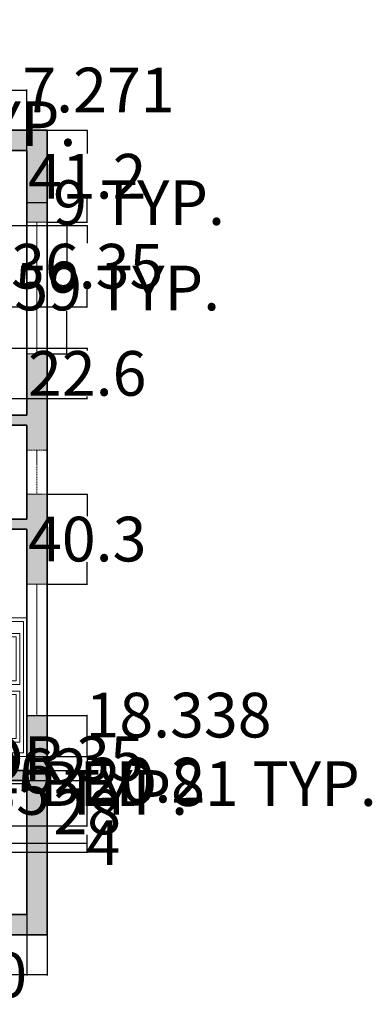
# Model space of a CAD drawing. Units: inches. Extents: x 305 to 776, y 38 to 479.
# Tile 14 of 14: x 618 to 776, y 38 to 479. Entities that reach past the tile are written whole.
import ezdxf

# ---------------------------------------------------------------- set-up
doc = ezdxf.new("R2010")
doc.units = ezdxf.units.IN
doc.header["$MEASUREMENT"] = 0
doc.linetypes.add('DASHED', pattern=[0.75, 0.5, -0.25])
for name, color, linetype, lineweight in [('A-ANNO-DIMS', 2, 'Continuous', 18), ('A-FURN', 8, 'Continuous', 18), ('A-GLAZ', 4, 'Continuous', 20), ('A-GLAZ-OVHD', 4, 'DASHED', 18), ('A-WALL', 7, 'Continuous', 35), ('A-WALL-PATT', 252, 'Continuous', 13)]:
    doc.layers.add(name, color=color, linetype=linetype, lineweight=lineweight)
doc.styles.get("Standard").update_dxf_attribs({"font": 'arial.ttf'})
doc.dimstyles.get("Standard").update_dxf_attribs({"dimtxt": 20, "dimasz": 0.18, "dimexe": 0.18, "dimexo": 0.0625, "dimgap": 0.09, "dimtad": 0, "dimtih": 1, "dimtoh": 1, "dimdec": 4, "dimzin": 0, "dimdsep": 46, "dimtxsty": 'Standard', "dimcen": 0.09, "dimadec": 0, "dimazin": 0, "dimtfac": 1, "dimtdec": 4, "dimtofl": 0, "dimtmove": 0, "dimatfit": 3, "dimfxl": 1, "dimtolj": 1, "dimtzin": 0, "dimarcsym": 0})

# ---------------------------------------------------------------- blocks, each defined once
blk = doc.blocks.new('W1')
blk.add_line((867.01, 338.44), (847.41, 338.44))
blk.add_lwpolyline([(847.41, 333.94), (867.01, 333.94), (867.01, 342.94), (847.41, 342.94)], close=True)
blk = doc.blocks.new('BED')
for p, q in [((1579.44, 254.58), (1564.49, 243.77)), ((1564.49, 243.77), (1579.44, 254.58)), ((1626.49, 254.58), (1579.44, 254.58)), ((1579.44, 254.58), (1579.44, 243.77)), ((1626.49, 253.76), (1579.44, 253.76)), ((1579.44, 243.77), (1564.49, 243.77))]:
    blk.add_line(p, q)
for points in [[(1626.49, 214.2), (1564.49, 214.2), (1564.49, 294.96), (1626.49, 294.96)], [(1624.92, 215.77), (1566.06, 215.77), (1566.06, 293.39), (1624.92, 293.39)], [(1594.24, 275.39), (1571.42, 275.39), (1571.42, 291.78), (1594.24, 291.78)], [(1620.04, 275.39), (1597.22, 275.39), (1597.22, 291.78), (1620.04, 291.78)], [(1592.67, 276.96), (1572.99, 276.96), (1572.99, 290.21), (1592.67, 290.21)], [(1618.47, 276.96), (1598.79, 276.96), (1598.79, 290.21), (1618.47, 290.21)]]:
    blk.add_lwpolyline(points, close=True)
blk = doc.blocks.new('W3')
for p, q in [((867.01, 308.31), (847.41, 308.31)), ((886.61, 308.31), (867.01, 308.31)), ((906.21, 308.31), (886.61, 308.31))]:
    blk.add_line(p, q)
for points in [[(867.01, 312.81), (847.41, 312.81), (847.41, 303.81), (867.01, 303.81)], [(886.61, 312.81), (867.01, 312.81)], [(886.61, 303.81), (906.21, 303.81), (906.21, 312.81), (886.61, 312.81)], [(867.01, 303.81), (886.61, 303.81)]]:
    blk.add_lwpolyline(points)
blk = doc.blocks.new('*D17')
at = {"layer": 'A-ANNO-DIMS', "color": 0, "lineweight": -2, "transparency": 16777216}
for p, q in [((476.73, 138.32), (476.73, 132.89)), ((512.13, 138.32), (512.13, 132.89)), ((476.91, 133.07), (511.95, 133.07)), ((512.13, 133.07), (512.31, 133.07))]:
    blk.add_line(p, q, dxfattribs=at)
at = {"layer": 'A-ANNO-DIMS', "color": 0, "transparency": 16777216}
for points in [[(476.91, 133.1), (476.91, 133.04), (476.73, 133.07)], [(511.95, 133.1), (511.95, 133.04), (512.13, 133.07)]]:
    blk.add_solid(points, dxfattribs=at)
at = {"layer": 'Defpoints', "color": 0, "transparency": 16777216}
for p in [(476.73, 138.38), (512.13, 138.38), (512.13, 133.07)]:
    blk.add_point(p, dxfattribs=at)
at = {"layer": 'A-ANNO-DIMS', "color": 0, "transparency": 16777216, "insert": (606.37, 133.07), "char_height": 20, "attachment_point": 5}
blk.add_mtext('\\A1;DOOR 35 TYP.', dxfattribs=at)
blk = doc.blocks.new('*D21')
at = {"layer": 'A-ANNO-DIMS', "color": 0, "lineweight": -2, "transparency": 16777216}
for p, q in [((403.93, 142.94), (403.93, 148.37)), ((404.11, 148.19), (439.15, 148.19)), ((439.33, 142.94), (439.33, 148.37)), ((439.33, 148.19), (439.51, 148.19))]:
    blk.add_line(p, q, dxfattribs=at)
at = {"layer": 'A-ANNO-DIMS', "color": 0, "transparency": 16777216}
for points in [[(404.11, 148.22), (404.11, 148.16), (403.93, 148.19)], [(439.15, 148.22), (439.15, 148.16), (439.33, 148.19)]]:
    blk.add_solid(points, dxfattribs=at)
at = {"layer": 'Defpoints', "color": 0, "transparency": 16777216}
for p in [(439.33, 148.19), (403.93, 142.88), (439.33, 142.88)]:
    blk.add_point(p, dxfattribs=at)
at = {"layer": 'A-ANNO-DIMS', "color": 0, "transparency": 16777216, "insert": (560.63, 148.19), "char_height": 20, "attachment_point": 5}
blk.add_mtext('\\A1;DOUBLE DOOR 35', dxfattribs=at)
blk = doc.blocks.new('*D23')
at = {"layer": 'A-ANNO-DIMS', "color": 0, "lineweight": -2, "transparency": 16777216}
for p, q in [((481.33, 429.44), (481.33, 432.5)), ((481.51, 432.32), (500.75, 432.32)), ((500.93, 429.44), (500.93, 432.5)), ((500.93, 432.32), (501.11, 432.32))]:
    blk.add_line(p, q, dxfattribs=at)
at = {"layer": 'A-ANNO-DIMS', "color": 0, "transparency": 16777216}
for points in [[(481.51, 432.35), (481.51, 432.29), (481.33, 432.32)], [(500.75, 432.35), (500.75, 432.29), (500.93, 432.32)]]:
    blk.add_solid(points, dxfattribs=at)
at = {"layer": 'Defpoints', "color": 0, "transparency": 16777216}
for p in [(500.93, 432.32), (481.33, 429.38), (500.93, 429.38)]:
    blk.add_point(p, dxfattribs=at)
at = {"layer": 'A-ANNO-DIMS', "color": 0, "transparency": 16777216, "insert": (575.13, 432.32), "char_height": 20, "attachment_point": 5}
blk.add_mtext('\\A1;W1 20 TYP.', dxfattribs=at)
blk = doc.blocks.new('*D27')
at = {"layer": 'A-ANNO-DIMS', "color": 0, "lineweight": -2, "transparency": 16777216}
for p, q in [((630.7, 388.18), (639.63, 388.18)), ((639.45, 388), (639.45, 369.09)), ((639.45, 329.56), (639.45, 348.47)), ((630.7, 329.38), (639.63, 329.38))]:
    blk.add_line(p, q, dxfattribs=at)
at = {"layer": 'A-ANNO-DIMS', "color": 0, "transparency": 16777216}
for points in [[(639.42, 388), (639.48, 388), (639.45, 388.18)], [(639.42, 329.56), (639.48, 329.56), (639.45, 329.38)]]:
    blk.add_solid(points, dxfattribs=at)
at = {"layer": 'Defpoints', "color": 0, "transparency": 16777216}
for p in [(630.63, 388.18), (630.63, 329.38), (639.45, 329.38)]:
    blk.add_point(p, dxfattribs=at)
at = {"layer": 'A-ANNO-DIMS', "color": 0, "transparency": 16777216, "insert": (639.45, 358.78), "char_height": 20, "attachment_point": 5}
blk.add_mtext('\\A1;W3 59 TYP.', dxfattribs=at)
blk = doc.blocks.new('*D28')
at = {"layer": 'A-ANNO-DIMS', "color": 0, "lineweight": -2, "transparency": 16777216}
for p, q in [((621.63, 388.24), (621.63, 397.18)), ((621.81, 397), (630.45, 397)), ((630.63, 388.24), (630.63, 397.18)), ((630.63, 397), (630.81, 397))]:
    blk.add_line(p, q, dxfattribs=at)
at = {"layer": 'A-ANNO-DIMS', "color": 0, "transparency": 16777216}
for points in [[(621.81, 397.03), (621.81, 396.97), (621.63, 397)], [(630.45, 397.03), (630.45, 396.97), (630.63, 397)]]:
    blk.add_solid(points, dxfattribs=at)
at = {"layer": 'Defpoints', "color": 0, "transparency": 16777216}
for p in [(630.63, 397), (621.63, 388.18), (630.63, 388.18)]:
    blk.add_point(p, dxfattribs=at)
at = {"layer": 'A-ANNO-DIMS', "color": 0, "transparency": 16777216, "insert": (671.81, 397), "char_height": 20, "attachment_point": 5}
blk.add_mtext('\\A1;9 TYP.', dxfattribs=at)
blk = doc.blocks.new('*D29')
at = {"layer": 'A-ANNO-DIMS', "color": 0, "lineweight": -2, "transparency": 16777216}
for p, q in [((540.87, 149.08), (540.87, 136.85)), ((621.63, 149.08), (621.63, 136.85)), ((541.05, 137.03), (621.45, 137.03)), ((621.63, 137.03), (621.81, 137.03))]:
    blk.add_line(p, q, dxfattribs=at)
at = {"layer": 'A-ANNO-DIMS', "color": 0, "transparency": 16777216}
for points in [[(541.05, 137.06), (541.05, 137), (540.87, 137.03)], [(621.45, 137.06), (621.45, 137), (621.63, 137.03)]]:
    blk.add_solid(points, dxfattribs=at)
at = {"layer": 'Defpoints', "color": 0, "transparency": 16777216}
for p in [(540.87, 149.14), (621.63, 149.14), (621.63, 137.03)]:
    blk.add_point(p, dxfattribs=at)
at = {"layer": 'A-ANNO-DIMS', "color": 0, "transparency": 16777216, "insert": (702.74, 137.03), "char_height": 20, "attachment_point": 5}
blk.add_mtext('\\A1;BED 81 TYP.', dxfattribs=at)
blk = doc.blocks.new('*D45')
at = {"layer": 'A-ANNO-DIMS', "color": 0, "lineweight": -2, "transparency": 16777216}
for p, q in [((390.63, 69.32), (390.63, 51.2)), ((630.63, 69.32), (630.63, 51.2)), ((390.81, 51.38), (488.31, 51.38)), ((630.45, 51.38), (532.95, 51.38))]:
    blk.add_line(p, q, dxfattribs=at)
at = {"layer": 'A-ANNO-DIMS', "color": 0, "transparency": 16777216}
for points in [[(390.81, 51.41), (390.81, 51.35), (390.63, 51.38)], [(630.45, 51.41), (630.45, 51.35), (630.63, 51.38)]]:
    blk.add_solid(points, dxfattribs=at)
at = {"layer": 'Defpoints', "color": 0, "transparency": 16777216}
for p in [(390.63, 69.38), (630.63, 69.38), (630.63, 51.38)]:
    blk.add_point(p, dxfattribs=at)
at = {"layer": 'A-ANNO-DIMS', "color": 0, "transparency": 16777216, "insert": (510.63, 51.38), "char_height": 20, "attachment_point": 5}
blk.add_mtext('\\A1;240', dxfattribs=at)
blk = doc.blocks.new('*D48')
at = {"layer": 'A-ANNO-DIMS', "color": 0, "lineweight": -2, "transparency": 16777216}
for p, q in [((404, 138.38), (648.81, 138.38)), ((648.63, 138.38), (648.63, 138.56)), ((648.63, 138.56), (648.81, 138.56)), ((648.63, 118.36), (648.63, 138.2)), ((399.7, 118.18), (648.81, 118.18))]:
    blk.add_line(p, q, dxfattribs=at)
at = {"layer": 'A-ANNO-DIMS', "color": 0, "transparency": 16777216}
for points in [[(648.6, 138.2), (648.66, 138.2), (648.63, 138.38)], [(648.6, 118.36), (648.66, 118.36), (648.63, 118.18)]]:
    blk.add_solid(points, dxfattribs=at)
at = {"layer": 'Defpoints', "color": 0, "transparency": 16777216}
for p in [(403.93, 138.38), (648.63, 138.38), (399.63, 118.18)]:
    blk.add_point(p, dxfattribs=at)
at = {"layer": 'A-ANNO-DIMS', "color": 0, "transparency": 16777216, "insert": (674.95, 138.56), "char_height": 20, "attachment_point": 5}
blk.add_mtext('\\A1;20.2', dxfattribs=at)
blk = doc.blocks.new('*D49')
at = {"layer": 'A-ANNO-DIMS', "color": 0, "lineweight": -2, "transparency": 16777216}
for p, q in [((399.7, 331.88), (648.81, 331.88)), ((648.63, 331.7), (648.63, 330.88)), ((399.7, 309.28), (648.81, 309.28)), ((648.63, 309.46), (648.63, 310.28))]:
    blk.add_line(p, q, dxfattribs=at)
at = {"layer": 'A-ANNO-DIMS', "color": 0, "transparency": 16777216}
for points in [[(648.6, 331.7), (648.66, 331.7), (648.63, 331.88)], [(648.6, 309.46), (648.66, 309.46), (648.63, 309.28)]]:
    blk.add_solid(points, dxfattribs=at)
at = {"layer": 'Defpoints', "color": 0, "transparency": 16777216}
for p in [(399.63, 331.88), (648.63, 331.88), (399.63, 309.28)]:
    blk.add_point(p, dxfattribs=at)
at = {"layer": 'A-ANNO-DIMS', "color": 0, "transparency": 16777216, "insert": (648.63, 320.58), "char_height": 20, "attachment_point": 5}
blk.add_mtext('\\A1;22.6', dxfattribs=at)
blk = doc.blocks.new('*D51')
at = {"layer": 'A-ANNO-DIMS', "color": 0, "lineweight": -2, "transparency": 16777216}
for p, q in [((621.7, 167.48), (648.81, 167.48)), ((648.63, 167.48), (648.63, 167.66)), ((648.63, 167.66), (648.81, 167.66)), ((648.63, 149.32), (648.63, 167.3)), ((621.7, 149.14), (648.81, 149.14))]:
    blk.add_line(p, q, dxfattribs=at)
at = {"layer": 'A-ANNO-DIMS', "color": 0, "transparency": 16777216}
for points in [[(648.6, 167.3), (648.66, 167.3), (648.63, 167.48)], [(648.6, 149.32), (648.66, 149.32), (648.63, 149.14)]]:
    blk.add_solid(points, dxfattribs=at)
at = {"layer": 'Defpoints', "color": 0, "transparency": 16777216}
for p in [(621.63, 167.48), (648.63, 167.48), (621.63, 149.14)]:
    blk.add_point(p, dxfattribs=at)
at = {"layer": 'A-ANNO-DIMS', "color": 0, "transparency": 16777216, "insert": (689.5, 167.66), "char_height": 20, "attachment_point": 5}
blk.add_mtext('\\A1;18.338', dxfattribs=at)
blk = doc.blocks.new('*D52')
at = {"layer": 'A-ANNO-DIMS', "color": 0, "lineweight": -2, "transparency": 16777216}
for p, q in [((630.7, 266.58), (648.81, 266.58)), ((648.63, 266.4), (648.63, 256.74)), ((648.63, 226.46), (648.63, 236.12)), ((630.7, 226.28), (648.81, 226.28))]:
    blk.add_line(p, q, dxfattribs=at)
at = {"layer": 'A-ANNO-DIMS', "color": 0, "transparency": 16777216}
for points in [[(648.6, 266.4), (648.66, 266.4), (648.63, 266.58)], [(648.6, 226.46), (648.66, 226.46), (648.63, 226.28)]]:
    blk.add_solid(points, dxfattribs=at)
at = {"layer": 'Defpoints', "color": 0, "transparency": 16777216}
for p in [(630.63, 266.58), (648.63, 266.58), (630.63, 226.28)]:
    blk.add_point(p, dxfattribs=at)
at = {"layer": 'A-ANNO-DIMS', "color": 0, "transparency": 16777216, "insert": (648.63, 246.43), "char_height": 20, "attachment_point": 5}
blk.add_mtext('\\A1;40.3', dxfattribs=at)
blk = doc.blocks.new('*D53')
at = {"layer": 'A-ANNO-DIMS', "color": 0, "lineweight": -2, "transparency": 16777216}
for p, q in [((630.7, 429.38), (648.81, 429.38)), ((648.63, 429.2), (648.63, 418.91)), ((648.63, 388.36), (648.63, 398.65)), ((630.7, 388.18), (648.81, 388.18))]:
    blk.add_line(p, q, dxfattribs=at)
at = {"layer": 'A-ANNO-DIMS', "color": 0, "transparency": 16777216}
for points in [[(648.6, 429.2), (648.66, 429.2), (648.63, 429.38)], [(648.6, 388.36), (648.66, 388.36), (648.63, 388.18)]]:
    blk.add_solid(points, dxfattribs=at)
at = {"layer": 'Defpoints', "color": 0, "transparency": 16777216}
for p in [(630.63, 429.38), (630.63, 388.18), (648.63, 388.18)]:
    blk.add_point(p, dxfattribs=at)
at = {"layer": 'A-ANNO-DIMS', "color": 0, "transparency": 16777216, "insert": (648.63, 408.78), "char_height": 20, "attachment_point": 5}
blk.add_mtext('\\A1;41.2', dxfattribs=at)
blk = doc.blocks.new('*D56')
at = {"layer": 'A-ANNO-DIMS', "color": 0, "lineweight": -2, "transparency": 16777216}
for p, q in [((591.63, 78.32), (591.63, 51.2)), ((621.63, 78.32), (621.63, 51.2)), ((591.81, 51.38), (592.26, 51.38)), ((621.45, 51.38), (621.01, 51.38))]:
    blk.add_line(p, q, dxfattribs=at)
at = {"layer": 'A-ANNO-DIMS', "color": 0, "transparency": 16777216}
for points in [[(591.81, 51.41), (591.81, 51.35), (591.63, 51.38)], [(621.45, 51.41), (621.45, 51.35), (621.63, 51.38)]]:
    blk.add_solid(points, dxfattribs=at)
at = {"layer": 'Defpoints', "color": 0, "transparency": 16777216}
for p in [(591.63, 78.38), (621.63, 78.38), (621.63, 51.38)]:
    blk.add_point(p, dxfattribs=at)
at = {"layer": 'A-ANNO-DIMS', "color": 0, "transparency": 16777216, "insert": (606.63, 51.38), "char_height": 20, "attachment_point": 5}
blk.add_mtext('\\A1;30', dxfattribs=at)
blk = doc.blocks.new('*D57')
at = {"layer": 'A-ANNO-DIMS', "color": 0, "lineweight": -2, "transparency": 16777216}
for p, q in [((591.7, 138.38), (648.81, 138.38)), ((648.63, 138.2), (648.63, 134.68)), ((591.7, 110.38), (648.81, 110.38)), ((648.63, 110.56), (648.63, 114.08))]:
    blk.add_line(p, q, dxfattribs=at)
at = {"layer": 'A-ANNO-DIMS', "color": 0, "transparency": 16777216}
for points in [[(648.6, 138.2), (648.66, 138.2), (648.63, 138.38)], [(648.6, 110.56), (648.66, 110.56), (648.63, 110.38)]]:
    blk.add_solid(points, dxfattribs=at)
at = {"layer": 'Defpoints', "color": 0, "transparency": 16777216}
for p in [(591.63, 138.38), (591.63, 110.38), (648.63, 110.38)]:
    blk.add_point(p, dxfattribs=at)
at = {"layer": 'A-ANNO-DIMS', "color": 0, "transparency": 16777216, "insert": (648.63, 124.38), "char_height": 20, "attachment_point": 5}
blk.add_mtext('\\A1;28', dxfattribs=at)
blk = doc.blocks.new('*D59')
at = {"layer": 'A-ANNO-DIMS', "color": 0, "lineweight": -2, "transparency": 16777216}
for p, q in [((591.7, 110.38), (648.81, 110.38)), ((648.63, 110.38), (648.63, 110.56)), ((648.63, 110.56), (648.81, 110.56)), ((648.63, 106.56), (648.63, 110.2)), ((591.7, 106.38), (648.81, 106.38))]:
    blk.add_line(p, q, dxfattribs=at)
at = {"layer": 'A-ANNO-DIMS', "color": 0, "transparency": 16777216}
for points in [[(648.6, 110.2), (648.66, 110.2), (648.63, 110.38)], [(648.6, 106.56), (648.66, 106.56), (648.63, 106.38)]]:
    blk.add_solid(points, dxfattribs=at)
at = {"layer": 'Defpoints', "color": 0, "transparency": 16777216}
for p in [(591.63, 110.38), (648.63, 110.38), (591.63, 106.38)]:
    blk.add_point(p, dxfattribs=at)
at = {"layer": 'A-ANNO-DIMS', "color": 0, "transparency": 16777216, "insert": (655.82, 110.56), "char_height": 20, "attachment_point": 5}
blk.add_mtext('\\A1;4', dxfattribs=at)
blk = doc.blocks.new('*D64')
at = {"layer": 'A-ANNO-DIMS', "color": 0, "lineweight": -2, "transparency": 16777216}
for p, q in [((400.62, 386.71), (648.81, 386.71)), ((648.63, 386.53), (648.63, 378.84)), ((648.63, 350.53), (648.63, 358.22)), ((400.62, 350.35), (648.81, 350.35))]:
    blk.add_line(p, q, dxfattribs=at)
at = {"layer": 'A-ANNO-DIMS', "color": 0, "transparency": 16777216}
for points in [[(648.6, 386.53), (648.66, 386.53), (648.63, 386.71)], [(648.6, 350.53), (648.66, 350.53), (648.63, 350.35)]]:
    blk.add_solid(points, dxfattribs=at)
at = {"layer": 'Defpoints', "color": 0, "transparency": 16777216}
for p in [(400.56, 386.71), (648.63, 386.71), (400.56, 350.35)]:
    blk.add_point(p, dxfattribs=at)
at = {"layer": 'A-ANNO-DIMS', "color": 0, "transparency": 16777216, "insert": (648.63, 368.53), "char_height": 20, "attachment_point": 5}
blk.add_mtext('\\A1;36.35', dxfattribs=at)
blk = doc.blocks.new('*D68')
at = {"layer": 'A-ANNO-DIMS', "color": 0, "lineweight": -2, "transparency": 16777216}
for p, q in [((614.36, 420.44), (614.36, 447.56)), ((614.54, 447.38), (621.45, 447.38)), ((621.63, 420.44), (621.63, 447.56)), ((621.63, 447.38), (621.81, 447.38))]:
    blk.add_line(p, q, dxfattribs=at)
at = {"layer": 'A-ANNO-DIMS', "color": 0, "transparency": 16777216}
for points in [[(614.54, 447.41), (614.54, 447.35), (614.36, 447.38)], [(621.45, 447.41), (621.45, 447.35), (621.63, 447.38)]]:
    blk.add_solid(points, dxfattribs=at)
at = {"layer": 'Defpoints', "color": 0, "transparency": 16777216}
for p in [(621.63, 447.38), (614.36, 420.38), (621.63, 420.38)]:
    blk.add_point(p, dxfattribs=at)
at = {"layer": 'A-ANNO-DIMS', "color": 0, "transparency": 16777216, "insert": (653.64, 447.38), "char_height": 20, "attachment_point": 5}
blk.add_mtext('\\A1;7.271', dxfattribs=at)
blk = doc.blocks.new('*D69')
at = {"layer": 'A-ANNO-DIMS', "color": 0, "lineweight": -2, "transparency": 16777216}
for p, q in [((621.7, 149.14), (648.81, 149.14)), ((648.63, 148.96), (648.63, 143.06)), ((621.7, 142.88), (648.81, 142.88)), ((648.63, 142.7), (648.45, 142.7)), ((648.63, 142.88), (648.63, 142.7))]:
    blk.add_line(p, q, dxfattribs=at)
at = {"layer": 'A-ANNO-DIMS', "color": 0, "transparency": 16777216}
for points in [[(648.6, 148.96), (648.66, 148.96), (648.63, 149.14)], [(648.6, 143.06), (648.66, 143.06), (648.63, 142.88)]]:
    blk.add_solid(points, dxfattribs=at)
at = {"layer": 'Defpoints', "color": 0, "transparency": 16777216}
for p in [(621.63, 149.14), (621.63, 142.88), (648.63, 142.88)]:
    blk.add_point(p, dxfattribs=at)
at = {"layer": 'A-ANNO-DIMS', "color": 0, "transparency": 16777216, "insert": (614.67, 142.7), "char_height": 20, "attachment_point": 5}
blk.add_mtext('\\A1;6.262', dxfattribs=at)

msp = doc.modelspace()

# ---------------------------------------------------------------- hatches: boundary and pattern name
at = {"layer": 'A-WALL-PATT'}
h = msp.add_hatch(color=256, dxfattribs=at)
h.dxf.hatch_style = 1
h.paths.add_polyline_path([(481.3329, 429.382), (390.6329, 429.382), (390.6329, 398.067), (399.6329, 398.067), (399.6329, 420.382), (465.6329, 420.382), (465.6329, 331.882), (470.1329, 331.882), (470.1329, 355.882), (512.1329, 355.882), (512.1329, 337.282), (512.1329, 337.282), (515.8592, 337.282), (516.6329, 337.282), (516.6329, 360.382), (513.3171, 360.382), (470.1329, 360.382), (470.1329, 420.382), (481.3329, 420.382)])
h.paths.add_polyline_path([(630.6329, 429.382), (500.9329, 429.382), (500.9329, 420.382), (502.8693, 420.382), (512.1329, 420.382), (512.1329, 391.882), (516.6329, 391.882), (516.6329, 420.382), (621.6329, 420.382), (621.6329, 388.182), (630.6329, 388.182)])
h.paths.add_polyline_path([(630.6329, 329.382), (621.6329, 329.382), (621.6329, 301.882), (512.1329, 301.882), (512.1329, 297.382), (515.8592, 297.382), (557.6329, 297.382), (621.6329, 297.382), (621.6329, 286.182), (630.6329, 286.182)])
h.paths.add_polyline_path([(630.6329, 266.582), (621.6329, 266.582), (621.6329, 255.382), (589.1329, 255.382), (589.1329, 250.882), (621.6329, 250.882), (621.6329, 226.282), (630.6329, 226.282)])
h.paths.add_polyline_path([(630.6329, 167.482), (621.6329, 167.482), (621.6329, 149.1444), (621.6329, 142.882), (516.6329, 142.882), (516.6329, 261.982), (512.1329, 261.982), (512.1329, 138.382), (621.6329, 138.382), (621.6329, 78.382), (512.1329, 78.382), (512.1329, 69.382), (630.6329, 69.382)])
h.paths.add_polyline_path([(464.1329, 138.382), (476.7329, 138.382), (476.7329, 142.1084), (476.7329, 142.882), (459.6329, 142.882), (459.6329, 78.382), (399.6329, 78.382), (399.6329, 98.582), (390.6329, 98.582), (390.6329, 69.382), (464.1329, 69.382)])
h.paths.add_polyline_path([(459.6329, 142.882), (439.3329, 142.882), (439.3329, 138.382), (459.6329, 138.382)], flags=17)
h.paths.add_polyline_path([(399.6329, 138.382), (403.9329, 138.382), (403.9329, 141.5545), (403.9329, 141.5545), (403.9329, 142.882), (399.6329, 142.882), (399.6329, 250.4819), (390.6329, 250.4819), (390.6329, 118.182), (399.6329, 118.182)])
h.paths.add_polyline_path([(399.6329, 331.882), (428.2629, 331.882), (428.2629, 336.382), (399.6329, 336.382), (399.6329, 358.697), (390.6329, 358.697), (390.6329, 309.2819), (399.6329, 309.2819)])

# ---------------------------------------------------------------- linework, layer by layer
at = {"layer": 'A-WALL'}
for p, q in [((621.6329, 420.382), (516.6329, 420.382)), ((621.6329, 336.382), (621.6329, 420.382)), ((621.6329, 301.882), (621.6329, 336.382)), ((621.6329, 301.882), (512.1329, 301.882)), ((621.6329, 297.382), (557.6329, 297.382)), ((621.6329, 297.382), (557.6329, 297.382)), ((621.6329, 255.382), (621.6329, 297.382)), ((621.6329, 255.382), (589.1329, 255.382)), ((621.6329, 250.882), (589.1329, 250.882)), ((621.6329, 142.882), (621.6329, 250.882)), ((621.6329, 142.882), (516.6329, 142.882)), ((621.6329, 138.382), (464.1329, 138.382)), ((621.6329, 78.382), (621.6329, 138.382)), ((512.1329, 78.382), (621.6329, 78.382))]:
    msp.add_line(p, q, dxfattribs=at)
msp.add_lwpolyline([(390.6329, 69.382), (630.6329, 69.382), (630.6329, 429.382), (390.6329, 429.382)], close=True, dxfattribs=at)

# ---------------------------------------------------------------- block references
at = {"layer": 'A-FURN', "rotation": 270}
msp.add_blockref('BED', (326.6739, 1775.6374), dxfattribs=at)
at = {"layer": 'A-GLAZ', "rotation": 270}
for p in [(317.8213, 1235.5942), (317.8213, 1073.6942)]:
    msp.add_blockref('W3', p, dxfattribs=at)
at = {"layer": 'A-GLAZ-OVHD', "rotation": 90}
msp.add_blockref('W1', (964.5758, -580.8301), dxfattribs=at)

# ---------------------------------------------------------------- dimensions: what is measured, and where the dimension line sits
at = {"layer": 'A-ANNO-DIMS'}
for base, p1, p2, text, picture, middle in [((500.9329, 432.322), (481.3329, 429.382), (500.9329, 429.382), 'W1 <> TYP.', '*D23', (575.1251, 432.322)), ((630.6329, 397.002), (621.6329, 388.182), (630.6329, 388.182), '<> TYP.', '*D28', (671.8101, 397.002)), ((439.3329, 148.192), (403.9329, 142.882), (439.3329, 142.882), 'DOUBLE DOOR <>', '*D21', (560.6261, 148.192)), ((621.6329, 137.0299), (540.8697, 149.1444), (621.6329, 149.1444), 'BED <> TYP.', '*D29', (702.7419, 137.0299)), ((512.1329, 133.072), (476.7329, 138.382), (512.1329, 138.382), 'DOOR <> TYP.', '*D17', (606.3729, 133.072))]:
    dim = msp.add_linear_dim(base=base, p1=p1, p2=p2, text=text, dimstyle='Standard', override={"dimdec": 0, "dimlfac": 1, "dimrnd": 0, "dimzin": 0, "dimdsep": 46, "dimlunit": 2}, dxfattribs=at)
    dim.commit()
    dim.dimension.update_dxf_attribs({"geometry": picture, "text_midpoint": middle})
for base, p1, p2, override, picture, middle in [((621.6329, 447.3835), (614.3616, 420.382), (621.6329, 420.382), {"dimdec": 3, "dimlfac": 1, "dimrnd": 0, "dimzin": 0, "dimdsep": 46, "dimlunit": 2}, '*D68', (653.6355, 447.3835)), ((621.6329, 51.3805), (591.6329, 78.382), (621.6329, 78.382), {"dimdec": 0, "dimlfac": 1, "dimrnd": 0, "dimzin": 0, "dimdsep": 46, "dimlunit": 2}, '*D56', (606.6329, 51.3805)), ((630.6329, 51.3805), (390.6329, 69.382), (630.6329, 69.382), {"dimdec": 0, "dimlfac": 1, "dimrnd": 0, "dimzin": 0, "dimdsep": 46, "dimlunit": 2}, '*D45', (510.6329, 51.3805))]:
    dim = msp.add_linear_dim(base=base, p1=p1, p2=p2, dimstyle='Standard', override=override, dxfattribs=at)
    dim.commit()
    dim.dimension.update_dxf_attribs({"geometry": picture, "text_midpoint": middle})
for base, p1, p2, override, picture, middle in [((648.6344, 388.182), (630.6329, 429.382), (630.6329, 388.182), {"dimdec": 1, "dimlfac": 1, "dimrnd": 0, "dimzin": 0, "dimdsep": 46, "dimlunit": 2}, '*D53', (648.6344, 408.782)), ((648.6344, 386.7066), (400.5603, 350.3541), (400.5603, 386.7066), {"dimdec": 2, "dimlfac": 1, "dimrnd": 0, "dimzin": 0, "dimdsep": 46, "dimlunit": 2}, '*D64', (648.6344, 368.5304)), ((648.6344, 331.882), (399.6329, 309.2819), (399.6329, 331.882), {"dimdec": 1, "dimlfac": 1, "dimrnd": 0, "dimzin": 0, "dimdsep": 46, "dimlunit": 2}, '*D49', (648.6344, 320.582)), ((648.6344, 266.582), (630.6329, 226.282), (630.6329, 266.582), {"dimdec": 1, "dimlfac": 1, "dimrnd": 0, "dimzin": 0, "dimdsep": 46, "dimlunit": 2}, '*D52', (648.6344, 246.432)), ((648.6344, 167.482), (621.6329, 149.1444), (621.6329, 167.482), {"dimdec": 3, "dimlfac": 1, "dimrnd": 0, "dimzin": 0, "dimdsep": 46, "dimlunit": 2}, '*D51', (689.4979, 167.662)), ((648.6344, 142.882), (621.6329, 149.1444), (621.6329, 142.882), {"dimdec": 3, "dimlfac": 1, "dimrnd": 0, "dimzin": 0, "dimdsep": 46, "dimlunit": 2}, '*D69', (614.6673, 142.702)), ((648.6344, 138.382), (399.6329, 118.182), (403.9329, 138.382), {"dimdec": 1, "dimlfac": 1, "dimrnd": 0, "dimzin": 0, "dimdsep": 46, "dimlunit": 2}, '*D48', (674.9481, 138.562)), ((648.6344, 110.382), (591.6329, 138.382), (591.6329, 110.382), {"dimdec": 0, "dimlfac": 1, "dimrnd": 0, "dimzin": 0, "dimdsep": 46, "dimlunit": 2}, '*D57', (648.6344, 124.382)), ((648.6344, 110.382), (591.6329, 106.382), (591.6329, 110.382), {"dimdec": 0, "dimlfac": 1, "dimrnd": 0, "dimzin": 0, "dimdsep": 46, "dimlunit": 2}, '*D59', (655.8212, 110.562))]:
    dim = msp.add_linear_dim(base=base, p1=p1, p2=p2, angle=90, dimstyle='Standard', override=override, dxfattribs=at)
    dim.commit()
    dim.dimension.update_dxf_attribs({"geometry": picture, "text_midpoint": middle})
dim = msp.add_linear_dim(base=(639.4529, 329.382), p1=(630.6329, 388.182), p2=(630.6329, 329.382), angle=270, text='W3 <> TYP.', dimstyle='Standard', override={"dimdec": 0, "dimlfac": 1, "dimrnd": 0, "dimzin": 0, "dimdsep": 46, "dimlunit": 2}, dxfattribs=at)
dim.commit()
dim.dimension.update_dxf_attribs({"geometry": '*D27', "text_midpoint": (639.4529, 358.782)})

doc.saveas('drawing.dxf')
